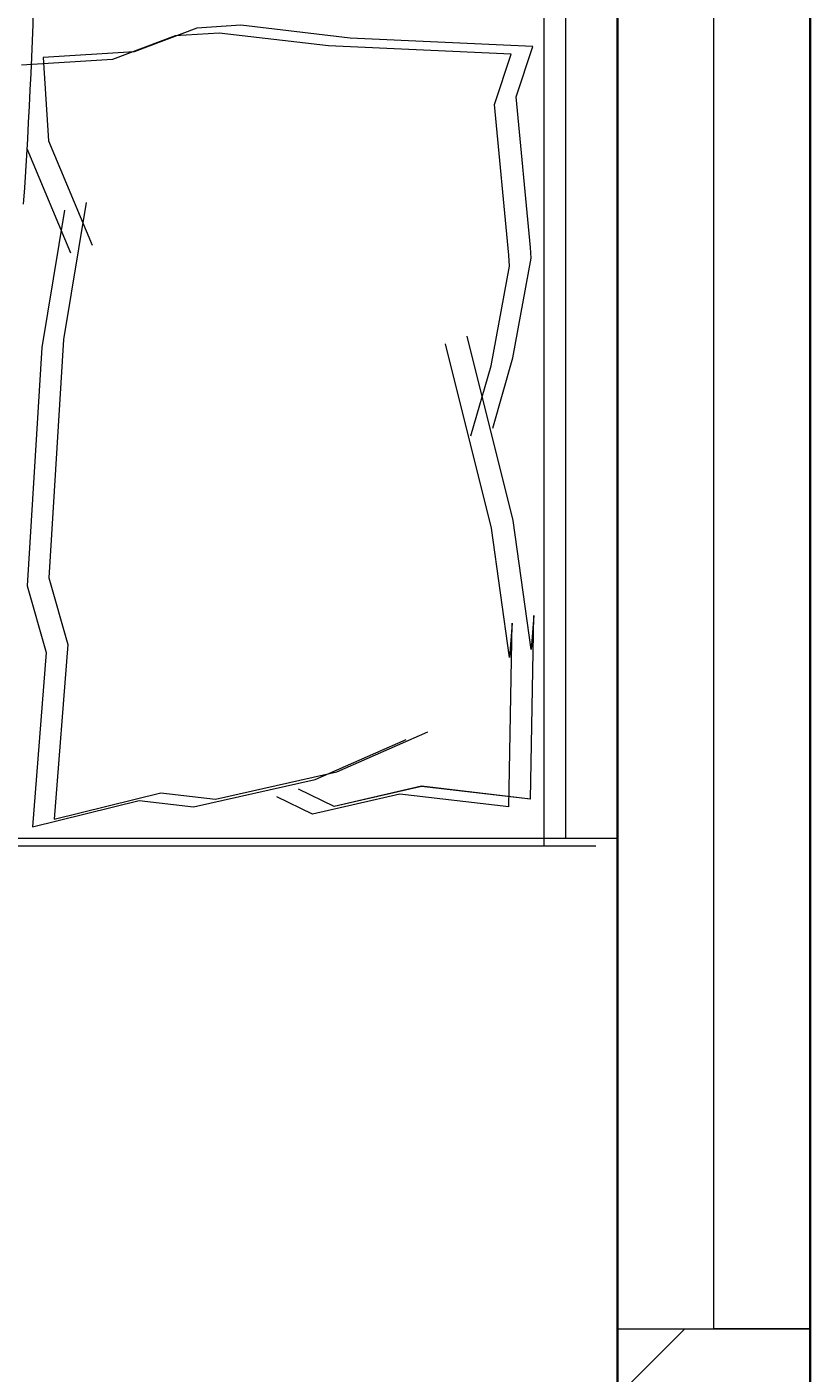
# Model space of a CAD drawing. Units: inches. Extents: x 1962 to 2771, y 1245 to 2660.
# Tile 75 of 114: x 2642 to 2661, y 2019 to 2051. Entities that reach past the tile are written whole.
import ezdxf

# ---------------------------------------------------------------- set-up
doc = ezdxf.new("R2010")
doc.units = ezdxf.units.IN
for name, color, linetype, lineweight in [('A-ANNO-DIMS', 2, 'Continuous', 18), ('A-FURN', 8, 'Continuous', 13), ('A-GLAZ', 4, 'Continuous', 18), ('A-WALL', 7, 'Continuous', 35), ('A-WALL-PATT', 252, 'Continuous', 13)]:
    doc.layers.add(name, color=color, linetype=linetype, lineweight=lineweight)
doc.styles.get("Standard").update_dxf_attribs({"font": 'arial.ttf'})
doc.dimstyles.get("Standard").update_dxf_attribs({"dimtxt": 0.18, "dimasz": 0.18, "dimexe": 0.18, "dimexo": 0.0625, "dimgap": 0.09, "dimtad": 0, "dimtih": 1, "dimtoh": 1, "dimdec": 4, "dimzin": 0, "dimdsep": 46, "dimtxsty": 'Standard', "dimcen": 0.09, "dimadec": 0, "dimazin": 0, "dimtfac": 1, "dimtdec": 4, "dimtofl": 0, "dimtmove": 0, "dimatfit": 3, "dimfxl": 1, "dimtolj": 1, "dimtzin": 0, "dimarcsym": 0})

# ---------------------------------------------------------------- blocks, each defined once
blk = doc.blocks.new('BED-PLAN')
for p, q in [((0.508, 40.933), (21.66, 40.933)), ((0.508, 40.933), (21.66, 40.933)), ((1.727, 2.945), (1.727, 40.933)), ((1.727, 2.945), (1.727, 40.933)), ((0, 40.752), (21.152, 40.752)), ((0, 40.751), (21.152, 40.751)), ((0, 2.764), (0, 40.751)), ((1.219, 2.764), (1.219, 40.752)), ((1.219, 2.763), (1.219, 40.751)), ((13.173, 40.301), (10.679, 39.684)), ((13.173, 40.301), (10.679, 39.684)), ((13.682, 40.482), (11.187, 39.866)), ((13.682, 40.482), (11.187, 39.866)), ((12.853, 36.222), (13.173, 40.301)), ((12.853, 36.221), (13.173, 40.301)), ((13.361, 36.403), (13.682, 40.482)), ((13.361, 36.403), (13.682, 40.482)), ((2.541, 40.016), (2.464, 35.722)), ((2.541, 40.016), (2.464, 35.722)), ((2.541, 40.016), (5.093, 39.715)), ((2.541, 40.016), (5.093, 39.715)), ((4.585, 39.534), (6.628, 40.007)), ((4.585, 39.533), (6.628, 40.007)), ((5.093, 39.715), (7.136, 40.188)), ((5.093, 39.715), (7.136, 40.188)), ((6.628, 40.007), (7.46, 39.598)), ((6.628, 40.007), (7.46, 39.598)), ((9.911, 40.016), (7.072, 39.378)), ((9.911, 40.016), (7.072, 39.378)), ((7.136, 40.188), (7.968, 39.78)), ((7.136, 40.188), (7.968, 39.78)), ((11.187, 39.866), (9.911, 40.016)), ((11.187, 39.866), (9.911, 40.016)), ((2.033, 39.835), (1.955, 35.54)), ((2.033, 39.834), (1.956, 35.54)), ((2.033, 39.835), (4.585, 39.534)), ((2.033, 39.834), (4.585, 39.533)), ((9.402, 39.835), (6.563, 39.197)), ((9.402, 39.835), (6.563, 39.197)), ((10.679, 39.684), (9.402, 39.835)), ((10.679, 39.684), (9.402, 39.835)), ((7.072, 39.378), (4.942, 38.439)), ((7.072, 39.378), (4.942, 38.439)), ((6.563, 39.197), (4.434, 38.258)), ((6.563, 39.197), (4.434, 38.258)), ((2.464, 35.722), (2.529, 36.519)), ((2.464, 35.722), (2.529, 36.519)), ((2.529, 36.519), (2.948, 33.5)), ((2.529, 36.519), (2.948, 33.5)), ((1.955, 35.54), (2.021, 36.338)), ((1.956, 35.54), (2.021, 36.337)), ((2.021, 36.338), (2.44, 33.319)), ((2.021, 36.337), (2.44, 33.318)), ((13.296, 34.663), (12.853, 36.222)), ((13.296, 34.663), (12.853, 36.221)), ((13.804, 34.845), (13.361, 36.403)), ((13.804, 34.845), (13.361, 36.403)), ((12.953, 29.091), (13.296, 34.663)), ((12.953, 29.091), (13.296, 34.663)), ((13.461, 29.273), (13.804, 34.845)), ((13.461, 29.273), (13.804, 34.845)), ((2.948, 33.5), (4.023, 29.192)), ((2.948, 33.5), (4.023, 29.192)), ((2.44, 33.319), (3.515, 29.011)), ((2.44, 33.318), (3.515, 29.011)), ((2.92, 31.161), (2.447, 29.52)), ((2.92, 31.161), (2.447, 29.519)), ((3.428, 31.343), (2.955, 29.701)), ((3.428, 31.342), (2.955, 29.701)), ((2.955, 29.701), (2.525, 27.372)), ((2.955, 29.701), (2.525, 27.372)), ((2.447, 29.52), (2.017, 27.19)), ((2.447, 29.519), (2.017, 27.19)), ((12.931, 26.068), (13.461, 29.273)), ((12.931, 26.068), (13.461, 29.273)), ((12.423, 25.886), (12.953, 29.091)), ((12.423, 25.886), (12.953, 29.091)), ((2.017, 27.19), (2.033, 26.935)), ((2.017, 27.19), (2.033, 26.935)), ((2.525, 27.372), (2.541, 27.117)), ((2.525, 27.372), (2.541, 27.116)), ((2.541, 27.117), (2.876, 23.597)), ((2.541, 27.116), (2.876, 23.597)), ((13.814, 24.626), (12.793, 27.067)), ((13.814, 24.626), (12.793, 27.066)), ((2.033, 26.935), (2.368, 23.415)), ((2.033, 26.935), (2.368, 23.415)), ((13.306, 24.444), (12.285, 26.885)), ((13.306, 24.444), (12.285, 26.885)), ((13.428, 22.495), (13.306, 24.444)), ((13.428, 22.495), (13.306, 24.444)), ((2.368, 23.415), (1.981, 22.24)), ((2.368, 23.415), (1.981, 22.24)), ((2.876, 23.597), (2.489, 22.421)), ((2.876, 23.597), (2.489, 22.421)), ((11.809, 22.543), (13.936, 22.676)), ((11.809, 22.543), (13.936, 22.676)), ((2.489, 22.421), (6.762, 22.228)), ((2.489, 22.421), (6.762, 22.228)), ((9.838, 21.81), (11.301, 22.362)), ((9.838, 21.81), (11.301, 22.362)), ((10.346, 21.991), (11.809, 22.543)), ((10.346, 21.991), (11.809, 22.543)), ((11.301, 22.362), (13.428, 22.495)), ((11.301, 22.362), (13.428, 22.495)), ((1.981, 22.24), (6.254, 22.046)), ((1.981, 22.24), (6.254, 22.046)), ((6.254, 22.046), (8.806, 21.745)), ((6.254, 22.046), (8.806, 21.745)), ((6.762, 22.228), (9.314, 21.927)), ((6.762, 22.228), (9.314, 21.927)), ((8.806, 21.745), (9.838, 21.81)), ((8.806, 21.745), (9.838, 21.81)), ((9.314, 21.927), (10.346, 21.991)), ((9.314, 21.927), (10.346, 21.991))]:
    blk.add_line(p, q)
blk.add_arc((144.711, 16.979), 131.131, 176.08655, 186.78213)
blk.add_arc((144.711, 16.979), 131.131, 176.08655, 186.78213)
blk = doc.blocks.new('WIN-60IN-A')
for p, q in [((0, 60), (4.5, 60)), ((4.5, 60), (2.25, 60)), ((2.25, 60), (2.25, 0))]:
    blk.add_line(p, q)
blk = doc.blocks.new('*D40')
at = {"layer": 'A-ANNO-DIMS', "color": 0, "lineweight": -2, "transparency": 16777216}
for p, q in [((2072.02, 2033.906), (2072.02, 2583.474)), ((2660.807, 2524.406), (2660.807, 2583.474)), ((2072.2, 2583.294), (2366.02, 2583.294)), ((2660.627, 2583.294), (2366.808, 2583.294))]:
    blk.add_line(p, q, dxfattribs=at)
at = {"layer": 'A-ANNO-DIMS', "color": 0, "transparency": 16777216}
for points in [[(2072.2, 2583.324), (2072.2, 2583.264), (2072.02, 2583.294)], [(2660.627, 2583.324), (2660.627, 2583.264), (2660.807, 2583.294)]]:
    blk.add_solid(points, dxfattribs=at)
at = {"layer": 'Defpoints', "color": 0, "transparency": 16777216}
for p in [(2660.807, 2583.294), (2660.807, 2524.344), (2072.02, 2033.844)]:
    blk.add_point(p, dxfattribs=at)
at = {"layer": 'A-ANNO-DIMS', "color": 0, "transparency": 16777216, "insert": (2366.414, 2583.294), "char_height": 0.18, "attachment_point": 5}
blk.add_mtext('\\A1;588.8', dxfattribs=at)

msp = doc.modelspace()

# ---------------------------------------------------------------- hatches: boundary and pattern name
at = {"layer": 'A-WALL-PATT'}
h = msp.add_hatch(dxfattribs=at)
h.set_pattern_fill('ANSI32', color=256)
h.paths.add_polyline_path([(2090.8074, 2467.3437), (2141.6481, 2467.3437), (2141.6481, 2469.5937), (2141.6481, 2471.8437), (2086.3074, 2471.8437), (2086.3074, 2422.5333), (2090.8074, 2422.5333)])
h.paths.add_polyline_path([(2282.7664, 2471.8437), (2204.8982, 2471.8437), (2204.8982, 2467.3437), (2234.8074, 2467.3437), (2234.8074, 2311.3437), (2228.7492, 2311.3437), (2228.7492, 2306.8437), (2234.8074, 2306.8437), (2331.9227, 2306.8437), (2331.9227, 2309.0937), (2331.9227, 2311.3437), (2239.3074, 2311.3437), (2239.3074, 2467.3437), (2282.7664, 2467.3437), (2282.7664, 2469.5937)])
h.paths.add_polyline_path([(2471.4531, 2519.8437), (2552.011, 2519.8437), (2564.3996, 2519.8437), (2564.3996, 2511.1389), (2568.8996, 2511.1389), (2568.8996, 2524.3437), (2466.9531, 2524.3437), (2466.9531, 2471.8437), (2450.0749, 2471.8437), (2446.4672, 2471.8437), (2446.4672, 2467.3437), (2450.0749, 2467.3437), (2475.9988, 2467.3437), (2475.9988, 2469.5937), (2475.9988, 2471.8437), (2471.4531, 2471.8437)])
h.paths.add_polyline_path([(2575.2231, 2469.5937), (2575.2231, 2471.8437), (2568.8996, 2471.8437), (2568.8996, 2487.1389), (2564.3996, 2487.1389), (2564.3996, 2471.8437), (2556.511, 2471.8437), (2499.2904, 2471.8437), (2499.2904, 2467.3437), (2507.8074, 2467.3437), (2507.8074, 2311.3437), (2414.863, 2311.3437), (2414.863, 2306.8437), (2512.3074, 2306.8437), (2517.0114, 2306.8437), (2517.0114, 2309.0937), (2517.0114, 2311.3437), (2512.3074, 2311.3437), (2512.3074, 2467.3437), (2575.2231, 2467.3437)])
h.paths.add_polyline_path([(2660.8074, 2471.8437), (2600.9602, 2471.8437), (2600.9602, 2467.3437), (2656.3074, 2467.3437), (2656.3074, 2432.5704), (2660.8074, 2432.5704)])
h.paths.add_polyline_path([(2660.8074, 2372.5704), (2656.3074, 2372.5704), (2656.3074, 2311.3437), (2600.276, 2311.3437), (2600.276, 2309.0937), (2600.276, 2306.8437), (2656.3074, 2306.8437), (2656.3074, 2296.2593), (2660.8074, 2296.2593)])
h.paths.add_polyline_path([(2572.3074, 2306.8437), (2577.1385, 2306.8437), (2577.1385, 2311.3437), (2551.082, 2311.3437), (2551.082, 2306.8437), (2567.8074, 2306.8437), (2567.8074, 2258.8437), (2540.0574, 2258.8437), (2540.0574, 2256.5937), (2540.0574, 2254.3437), (2567.8074, 2254.3437), (2656.3074, 2254.3437), (2656.3074, 2236.9085), (2660.8074, 2236.9085), (2660.8074, 2272.2593), (2656.3074, 2272.2593), (2656.3074, 2258.8437), (2572.3074, 2258.8437)])
h.paths.add_polyline_path([(2512.3074, 2254.3437), (2518.8716, 2254.3437), (2518.8716, 2256.5937), (2518.8716, 2258.8437), (2507.8074, 2258.8437), (2507.8074, 2177.8437), (2567.8074, 2177.8437), (2567.8074, 2172.9628), (2572.3074, 2172.9628), (2572.3074, 2177.8437), (2656.3074, 2177.8437), (2656.3074, 2166.4846), (2660.8074, 2166.4846), (2660.8074, 2200.9085), (2656.3074, 2200.9085), (2656.3074, 2182.3437), (2512.3074, 2182.3437)])
h.paths.add_polyline_path([(2656.3074, 2129.8437), (2572.3074, 2129.8437), (2572.3074, 2150.3044), (2570.0574, 2150.3044), (2567.8074, 2150.3044), (2567.8074, 2129.8437), (2507.8074, 2129.8437), (2507.8074, 2116.3027), (2510.0574, 2116.3027), (2512.3074, 2116.3027), (2512.3074, 2125.3437), (2567.8074, 2125.3437), (2572.3074, 2125.3437), (2656.3074, 2125.3437)])
h.paths.add_polyline_path([(2090.8074, 2362.5333), (2086.3074, 2362.5333), (2086.3074, 2298.6242), (2090.8074, 2298.6242), (2090.8074, 2306.8437), (2174.8074, 2306.8437), (2174.8074, 2286.4178), (2179.3074, 2286.4178), (2179.3074, 2306.8437), (2192.8641, 2306.8437), (2192.8641, 2309.0937), (2192.8641, 2311.3437), (2090.8074, 2311.3437)])
h.paths.add_polyline_path([(2209.156, 2258.8437), (2179.3074, 2258.8437), (2179.3074, 2263.2236), (2177.0574, 2263.2236), (2174.8074, 2263.2236), (2174.8074, 2258.8437), (2090.8074, 2258.8437), (2090.8074, 2274.6242), (2086.3074, 2274.6242), (2086.3074, 2238.2967), (2088.5574, 2238.2967), (2090.8074, 2238.2967), (2090.8074, 2254.3437), (2209.156, 2254.3437)])
h.paths.add_polyline_path([(2090.8074, 2177.8437), (2234.8074, 2177.8437), (2234.8074, 2173.1428), (2239.3074, 2173.1428), (2239.3074, 2258.8437), (2230.8442, 2258.8437), (2230.8442, 2256.5937), (2230.8442, 2254.3437), (2234.8074, 2254.3437), (2234.8074, 2182.3437), (2090.8074, 2182.3437), (2090.8074, 2202.2967), (2086.3074, 2202.2967), (2086.3074, 2140.0389), (2090.8074, 2140.0389)])
h.paths.add_polyline_path([(2090.8074, 2080.0389), (2086.3074, 2080.0389), (2086.3074, 2033.8437), (2090.8074, 2033.8437)], flags=17)
h.paths.add_polyline_path([(2244.9405, 2033.8437), (2239.3074, 2033.8437), (2239.3074, 2142.0665), (2237.2592, 2142.0665), (2234.8074, 2142.0665), (2234.8074, 2033.8437), (2090.8074, 2033.8437), (2076.5204, 2033.8437), (2072.0204, 2033.8437), (2072.0204, 2000.4493), (2076.5204, 2000.4493), (2076.5204, 2029.3437), (2090.8074, 2029.3437), (2244.9405, 2029.3437), (2244.9405, 2031.5937)])
h.paths.add_polyline_path([(2234.8074, 1933.3437), (2076.5204, 1933.3437), (2076.5204, 1952.4493), (2074.2704, 1952.4493), (2072.0204, 1952.4493), (2072.0204, 1933.3437), (2072.0204, 1928.8437), (2234.8074, 1928.8437)])
h.paths.add_polyline_path([(2090.8074, 1928.8437), (2086.3074, 1928.8437), (2086.3074, 1906.5013), (2090.8074, 1906.5013)])
h.paths.add_polyline_path([(2090.8074, 1846.5013), (2086.3074, 1846.5013), (2086.3074, 1769.9917), (2088.5574, 1769.9917), (2090.8074, 1769.9917), (2090.8074, 1780.3437), (2234.8074, 1780.3437), (2234.8074, 1708.3437), (2230.3764, 1708.3437), (2230.3764, 1703.8437), (2239.3074, 1703.8437), (2239.3074, 1792.6669), (2237.0574, 1792.6669), (2234.8074, 1792.6669), (2234.8074, 1784.8437), (2090.8074, 1784.8437)])
h.paths.add_polyline_path([(2239.3074, 1928.8437), (2244.9405, 1928.8437), (2244.9405, 1931.0937), (2244.9405, 1933.3437), (2234.8074, 1933.3437), (2234.8074, 1928.8437), (2234.8074, 1825.5949), (2239.3074, 1825.5949)])
h.paths.add_polyline_path([(2148.0425, 1649.0937), (2148.0425, 1651.3437), (2090.8074, 1651.3437), (2090.8074, 1646.8437), (2148.0425, 1646.8437)], flags=0)
h.paths.add_polyline_path([(2207.5601, 1708.3437), (2090.8074, 1708.3437), (2090.8074, 1703.8437), (2174.8074, 1703.8437), (2174.8074, 1651.3437), (2170.4457, 1651.3437), (2170.4457, 1646.8437), (2195.9924, 1646.8437), (2195.9924, 1649.0937), (2195.9924, 1651.3437), (2179.3074, 1651.3437), (2179.3074, 1703.8437), (2207.5601, 1703.8437), (2207.5601, 1706.0937)])
h.paths.add_polyline_path([(2090.8074, 1733.9917), (2086.3074, 1733.9917), (2086.3074, 1696.1032), (2088.5574, 1696.1032), (2090.8074, 1696.1032)])
h.paths.add_polyline_path([(2090.8074, 1672.1032), (2086.3074, 1672.1032), (2086.3074, 1600.3335), (2090.8074, 1600.3335)])
h.paths.add_polyline_path([(2090.8074, 1540.3335), (2086.3074, 1540.3335), (2086.3074, 1486.3437), (2139.6766, 1486.3437), (2139.6766, 1490.8437), (2090.8074, 1490.8437)])
h.paths.add_polyline_path([(2302.3876, 1490.8437), (2239.3074, 1490.8437), (2239.3074, 1646.8437), (2335.9994, 1646.8437), (2335.9994, 1651.3437), (2229.884, 1651.3437), (2229.884, 1646.8437), (2234.8074, 1646.8437), (2234.8074, 1490.8437), (2202.7103, 1490.8437), (2202.7103, 1488.5937), (2202.7103, 1486.3437), (2275.0699, 1486.3437), (2275.0699, 1475.772), (2279.5699, 1475.772), (2279.5699, 1486.3437), (2302.3876, 1486.3437)])
h.paths.add_polyline_path([(2279.5699, 1451.772), (2275.0699, 1451.772), (2275.0699, 1438.3437), (2174.8074, 1438.3437), (2174.8074, 1486.3437), (2179.7922, 1486.3437), (2179.7922, 1490.8437), (2163.3585, 1490.8437), (2163.3585, 1488.5937), (2163.3585, 1486.3437), (2170.3074, 1486.3437), (2170.3074, 1433.8437), (2279.5699, 1433.8437)])
h.paths.add_polyline_path([(2427.2363, 1490.8437), (2375.8074, 1490.8437), (2375.8074, 1646.8437), (2381.6401, 1646.8437), (2381.6401, 1651.3437), (2365.887, 1651.3437), (2365.887, 1649.0937), (2365.887, 1646.8437), (2371.3074, 1646.8437), (2371.3074, 1490.8437), (2327.5627, 1490.8437), (2327.5627, 1488.5937), (2327.5627, 1486.3437), (2371.3074, 1486.3437), (2371.3074, 1433.8437), (2375.8074, 1433.8437), (2375.8074, 1486.3437), (2427.2363, 1486.3437)])
h.paths.add_polyline_path([(2512.3074, 1646.8437), (2519.4351, 1646.8437), (2519.4351, 1649.0937), (2519.4351, 1651.3437), (2507.8074, 1651.3437), (2416.0063, 1651.3437), (2416.0063, 1649.0937), (2416.0063, 1646.8437), (2507.8074, 1646.8437), (2507.8074, 1490.8437), (2497.0532, 1490.8437), (2497.0532, 1488.5937), (2497.0532, 1486.3437), (2574.9344, 1486.3437), (2574.9344, 1476.0181), (2579.4344, 1476.0181), (2579.4344, 1486.3437), (2584.4872, 1486.3437), (2584.3074, 1490.8437), (2512.3074, 1490.8437)])
h.paths.add_polyline_path([(2470.5091, 1486.3437), (2473.9767, 1486.3437), (2473.9767, 1490.8437), (2449.6605, 1490.8437), (2449.6605, 1488.5937), (2449.6605, 1486.3437), (2466.0091, 1486.3437), (2466.0091, 1433.8437), (2470.5091, 1433.8437), (2579.4344, 1433.8437), (2579.4344, 1452.0181), (2574.9344, 1452.0181), (2574.9344, 1438.3437), (2554.5091, 1438.3437), (2470.5091, 1438.3437)])
h.paths.add_polyline_path([(2656.3074, 1490.8437), (2611.86, 1490.8437), (2611.86, 1486.3437), (2656.3074, 1486.3437)])
h.paths.add_polyline_path([(2660.8074, 1532.7007), (2658.5574, 1532.7007), (2656.3074, 1532.7007), (2656.3074, 1486.3437), (2660.8074, 1486.3437)])
h.paths.add_polyline_path([(2660.8074, 1664.9663), (2656.3074, 1664.9663), (2656.3074, 1651.3437), (2602.2313, 1651.3437), (2602.2313, 1646.8437), (2656.3074, 1646.8437), (2656.3074, 1592.7007), (2660.8074, 1592.7007)])
h.paths.add_polyline_path([(2660.8074, 1724.5221), (2656.3074, 1724.5221), (2656.3074, 1703.8437), (2542.4725, 1703.8437), (2542.4725, 1699.3437), (2567.8074, 1699.3437), (2567.8074, 1651.3437), (2552.7766, 1651.3437), (2552.7766, 1649.0937), (2552.7766, 1646.8437), (2577.2878, 1646.8437), (2577.2878, 1649.0937), (2577.2878, 1651.3437), (2572.3074, 1651.3437), (2572.3074, 1699.3437), (2656.3074, 1699.3437), (2656.3074, 1688.9663), (2660.8074, 1688.9663)])
h.paths.add_polyline_path([(2660.8074, 1880.6524), (2656.3074, 1880.6524), (2656.3074, 1832.8437), (2512.3074, 1832.8437), (2512.3074, 1837.8959), (2507.8074, 1837.8959), (2507.8074, 1828.3437), (2567.8074, 1828.3437), (2567.8074, 1804.3437), (2572.3074, 1804.3437), (2572.3074, 1828.3437), (2656.3074, 1828.3437), (2656.3074, 1818.6778), (2660.8074, 1818.6778)])
h.paths.add_polyline_path([(2660.8074, 1794.6778), (2656.3074, 1794.6778), (2656.3074, 1780.3437), (2572.3074, 1780.3437), (2572.3074, 1783.0303), (2570.0574, 1783.0303), (2567.8074, 1783.0303), (2567.8074, 1780.3437), (2507.8074, 1780.3437), (2507.8074, 1699.3437), (2517.8858, 1699.3437), (2517.8858, 1701.5937), (2517.8858, 1703.8437), (2512.3074, 1703.8437), (2512.3074, 1775.8437), (2656.3074, 1775.8437), (2656.3074, 1760.5221), (2660.8074, 1760.5221)])
h.paths.add_polyline_path([(2660.8074, 1981.3437), (2660.8074, 2020.2808), (2658.5574, 2020.2808), (2656.3074, 2020.2808), (2656.3074, 1981.3437), (2512.3074, 1981.3437), (2512.3074, 2086.6996), (2507.8074, 2086.6996), (2507.8074, 1981.3437), (2375.8074, 1981.3437), (2375.8074, 1986.8505), (2373.5574, 1986.8505), (2371.3074, 1986.8505), (2371.3074, 1973.2607), (2375.8074, 1973.2607), (2375.8074, 1976.8437), (2507.8074, 1976.8437), (2507.8074, 1865.4281), (2510.0574, 1865.4281), (2512.3074, 1865.4281), (2512.3074, 1976.8437), (2660.8074, 1976.8437)])
h.paths.add_polyline_path([(2375.8074, 1940.297), (2373.5574, 1940.297), (2371.3074, 1940.297), (2371.3074, 1933.3437), (2278.4434, 1933.3437), (2278.4434, 1928.8437), (2371.3074, 1928.8437), (2371.3074, 1651.3437), (2375.8074, 1651.3437)])
h.paths.add_polyline_path([(2660.8074, 1976.8437), (2656.3074, 1976.8437), (2656.3074, 1940.6524), (2660.8074, 1940.6524)], flags=17)
h.paths.add_polyline_path([(2660.8074, 2142.4846), (2656.3074, 2142.4846), (2656.3074, 2080.2808), (2660.8074, 2080.2808)])
h.paths.add_polyline_path([(2381.4189, 2311.3437), (2375.8074, 2311.3437), (2375.8074, 2467.3437), (2424.7242, 2467.3437), (2424.7242, 2469.5937), (2424.7242, 2471.8437), (2375.8074, 2471.8437), (2375.8074, 2524.3437), (2371.3074, 2524.3437), (2371.3074, 2471.8437), (2307.2097, 2471.8437), (2307.2097, 2467.3437), (2371.3074, 2467.3437), (2371.3074, 2311.3437), (2366.8901, 2311.3437), (2366.8901, 2306.8437), (2371.3074, 2306.8437), (2371.3074, 2033.8437), (2279.6589, 2033.8437), (2279.6589, 2029.3437), (2371.3074, 2029.3437), (2371.3074, 2014.2598), (2375.8074, 2014.2598), (2375.8074, 2306.8437), (2381.4189, 2306.8437)])
h.paths.add_polyline_path([(2263.3074, 2524.3437), (2170.3074, 2524.3437), (2170.3074, 2519.8437), (2170.3074, 2471.8437), (2165.0312, 2471.8437), (2165.0312, 2467.3437), (2179.6721, 2467.3437), (2179.6721, 2469.5161), (2179.6721, 2471.8437), (2174.8074, 2471.8437), (2174.8074, 2519.8437), (2258.8074, 2519.8437), (2258.8074, 2511.6436), (2263.3074, 2511.6436)])
h.paths.add_polyline_path([(2245.0232, 1361.4123), (2492.9468, 1361.4123), (2492.9468, 1398.505), (2245.0232, 1398.505)], flags=9)
h.paths.add_polyline_path([(2388.1434, 2086.6936), (2425.0704, 2086.6936), (2425.0704, 2105.3509), (2388.1434, 2105.3509)], flags=9)
h.paths.add_polyline_path([(2404.922, 2242.6744), (2445.7337, 2242.6744), (2445.7337, 2261.3318), (2404.922, 2261.3318)], flags=9)
h.paths.add_polyline_path([(2269.4107, 2156.7935), (2306.3378, 2156.7935), (2306.3378, 2175.4508), (2269.4107, 2175.4508)], flags=9)
h.paths.add_polyline_path([(2269.3277, 2233.4343), (2306.2547, 2233.4343), (2306.2547, 2252.0917), (2269.3277, 2252.0917)], flags=9)
h.paths.add_polyline_path([(2431.6052, 2320.6922), (2470.4456, 2320.6922), (2470.4456, 2339.3495), (2431.6052, 2339.3495)], flags=25)
h.paths.add_polyline_path([(2249.6902, 2315.7608), (2288.5306, 2315.7608), (2288.5306, 2334.4182), (2249.6902, 2334.4182)], flags=25)
h.paths.add_polyline_path([(2096.9301, 2314.3181), (2135.7704, 2314.3181), (2135.7704, 2332.9755), (2096.9301, 2332.9755)], flags=25)
h.paths.add_polyline_path([(2134.3475, 2285.7089), (2161.4655, 2285.7089), (2161.4655, 2304.3662), (2134.3475, 2304.3662)], flags=9)
h.paths.add_polyline_path([(2126.5155, 2209.4076), (2159.9227, 2209.4076), (2159.9227, 2228.065), (2126.5155, 2228.065)], flags=25)
h.paths.add_polyline_path([(2110.5753, 2141.5299), (2149.4157, 2141.5299), (2149.4157, 2160.1872), (2110.5753, 2160.1872)], flags=25)
h.paths.add_polyline_path([(2249.8618, 1968.3317), (2286.3966, 1968.3317), (2286.3966, 1986.989), (2249.8618, 1986.989)], flags=9)
h.paths.add_polyline_path([(2395.9507, 1777.0051), (2436.7624, 1777.0051), (2436.7624, 1795.6625), (2395.9507, 1795.6625)], flags=9)
h.paths.add_polyline_path([(2398.5259, 1888.5651), (2435.0062, 1888.5651), (2435.0062, 1907.2224), (2398.5259, 1907.2224)], flags=25)
h.paths.add_polyline_path([(2259.3506, 1728.3559), (2296.2776, 1728.3559), (2296.2776, 1747.0132), (2259.3506, 1747.0132)], flags=9)
h.paths.add_polyline_path([(2271.3698, 1845.268), (2308.2968, 1845.268), (2308.2968, 1863.9253), (2271.3698, 1863.9253)], flags=9)
h.paths.add_polyline_path([(2120.9355, 1786.3027), (2159.7759, 1786.3027), (2159.7759, 1804.9601), (2120.9355, 1804.9601)], flags=25)
h.paths.add_polyline_path([(2121.3164, 1732.1043), (2154.7236, 1732.1043), (2154.7236, 1750.7616), (2121.3164, 1750.7616)], flags=25)
h.paths.add_polyline_path([(2118.3706, 1678.8997), (2147.5282, 1678.8997), (2147.5282, 1697.557), (2118.3706, 1697.557)], flags=25)
h.paths.add_polyline_path([(2385.9227, 1493.557), (2424.763, 1493.557), (2424.763, 1512.2143), (2385.9227, 1512.2143)], flags=25)
h.paths.add_polyline_path([(2248.7058, 1500.0256), (2287.5462, 1500.0256), (2287.5462, 1518.6829), (2248.7058, 1518.6829)], flags=25)
h.paths.add_polyline_path([(2104.1669, 1617.3771), (2143.0073, 1617.3771), (2143.0073, 1636.0344), (2104.1669, 1636.0344)], flags=9)
h.paths.add_polyline_path([(2096.0714, 1447.8824), (2137.3845, 1447.8824), (2137.3845, 1458.1859), (2096.0714, 1458.1859)], flags=9)
h.paths.add_polyline_path([(2180.6114, 1440.325), (2209.7689, 1440.325), (2209.7689, 1458.9823), (2180.6114, 1458.9823)], flags=25)
h.paths.add_polyline_path([(2316.1698, 1447.9637), (2357.4829, 1447.9637), (2357.4829, 1458.2673), (2316.1698, 1458.2673)], flags=9)
h.paths.add_polyline_path([(2397.6187, 1447.9637), (2438.9318, 1447.9637), (2438.9318, 1458.2673), (2397.6187, 1458.2673)], flags=9)
h.paths.add_polyline_path([(2473.0778, 1439.5953), (2502.2354, 1439.5953), (2502.2354, 1458.2527), (2473.0778, 1458.2527)], flags=25)
h.paths.add_polyline_path([(2589.7027, 1447.8819), (2631.0158, 1447.8819), (2631.0158, 1458.1855), (2589.7027, 1458.1855)], flags=9)
h.paths.add_polyline_path([(2522.4009, 1497.5285), (2561.2413, 1497.5285), (2561.2413, 1516.1859), (2522.4009, 1516.1859)], flags=25)
h.paths.add_polyline_path([(2579.6565, 1671.3482), (2608.8141, 1671.3482), (2608.8141, 1690.0056), (2579.6565, 1690.0056)], flags=25)
h.paths.add_polyline_path([(2544.7038, 1725.5064), (2578.1111, 1725.5064), (2578.1111, 1744.1637), (2544.7038, 1744.1637)], flags=25)
h.paths.add_polyline_path([(2578.1191, 1807.472), (2607.2766, 1807.472), (2607.2766, 1826.1293), (2578.1191, 1826.1293)], flags=25)
h.paths.add_polyline_path([(2595.0614, 1835.1839), (2633.9018, 1835.1839), (2633.9018, 1853.8413), (2595.0614, 1853.8413)], flags=25)
h.paths.add_polyline_path([(2567.0097, 2097.7035), (2605.8501, 2097.7035), (2605.8501, 2116.3609), (2567.0097, 2116.3609)], flags=9)
h.paths.add_polyline_path([(2586.644, 2134.6454), (2615.8015, 2134.6454), (2615.8015, 2153.3027), (2586.644, 2153.3027)], flags=9)
h.paths.add_polyline_path([(2544.6185, 2212.6783), (2578.0258, 2212.6783), (2578.0258, 2231.3356), (2544.6185, 2231.3356)], flags=25)
h.paths.add_polyline_path([(2577.0273, 2256.9023), (2606.1849, 2256.9023), (2606.1849, 2275.5597), (2577.0273, 2275.5597)], flags=24)
h.paths.add_polyline_path([(2605.2683, 2315.2821), (2644.1087, 2315.2821), (2644.1087, 2333.9395), (2605.2683, 2333.9395)], flags=25)
h.paths.add_polyline_path([(2583.1244, 2496.1815), (2624.4375, 2496.1815), (2624.4375, 2506.4851), (2583.1244, 2506.4851)], flags=9)
h.paths.add_polyline_path([(2474.761, 2497.0823), (2503.9185, 2497.0823), (2503.9185, 2515.7397), (2474.761, 2515.7397)], flags=25)
h.paths.add_polyline_path([(2387.5787, 2494.2563), (2428.902, 2494.2563), (2428.902, 2504.5598), (2387.5787, 2504.5598)], flags=9)
h.paths.add_polyline_path([(2300.1657, 2500.1564), (2341.4788, 2500.1564), (2341.4788, 2510.46), (2300.1657, 2510.46)], flags=25)
h.paths.add_polyline_path([(2176.8589, 2497.5843), (2206.0165, 2497.5843), (2206.0165, 2516.2416), (2176.8589, 2516.2416)], flags=25)
h.paths.add_polyline_path([(2097.4668, 2494.9762), (2138.7799, 2494.9762), (2138.7799, 2505.2798), (2097.4668, 2505.2798)], flags=9)

# ---------------------------------------------------------------- linework, layer by layer
at = {"layer": 'A-WALL'}
for p, q in [((2660.8074, 2471.8437), (2660.8074, 1976.8437)), ((2656.3074, 2177.8437), (2656.3074, 1981.3437))]:
    msp.add_line(p, q, dxfattribs=at)

# ---------------------------------------------------------------- block references
at = {"layer": 'A-FURN', "rotation": 180}
msp.add_blockref('BED-PLAN', (2656.3074, 2072.498), dxfattribs=at)
at = {"layer": 'A-GLAZ', "extrusion": (0, 0, -1), "zscale": -1, "rotation": 180}
msp.add_blockref('WIN-60IN-A', (-2656.3074, 2080.2808), dxfattribs=at)

# ---------------------------------------------------------------- dimensions: what is measured, and where the dimension line sits
at = {"layer": 'A-ANNO-DIMS'}
dim = msp.add_linear_dim(base=(2660.8074, 2583.2937), p1=(2072.0204, 2033.8437), p2=(2660.8074, 2524.3437), dimstyle='Standard', override={"dimdec": 1, "dimlfac": 1, "dimrnd": 0, "dimzin": 0, "dimdsep": 46, "dimlunit": 2}, dxfattribs=at)
dim.commit()
dim.dimension.update_dxf_attribs({"geometry": '*D40', "text_midpoint": (2366.4139, 2583.2937)})

doc.saveas('drawing.dxf')
